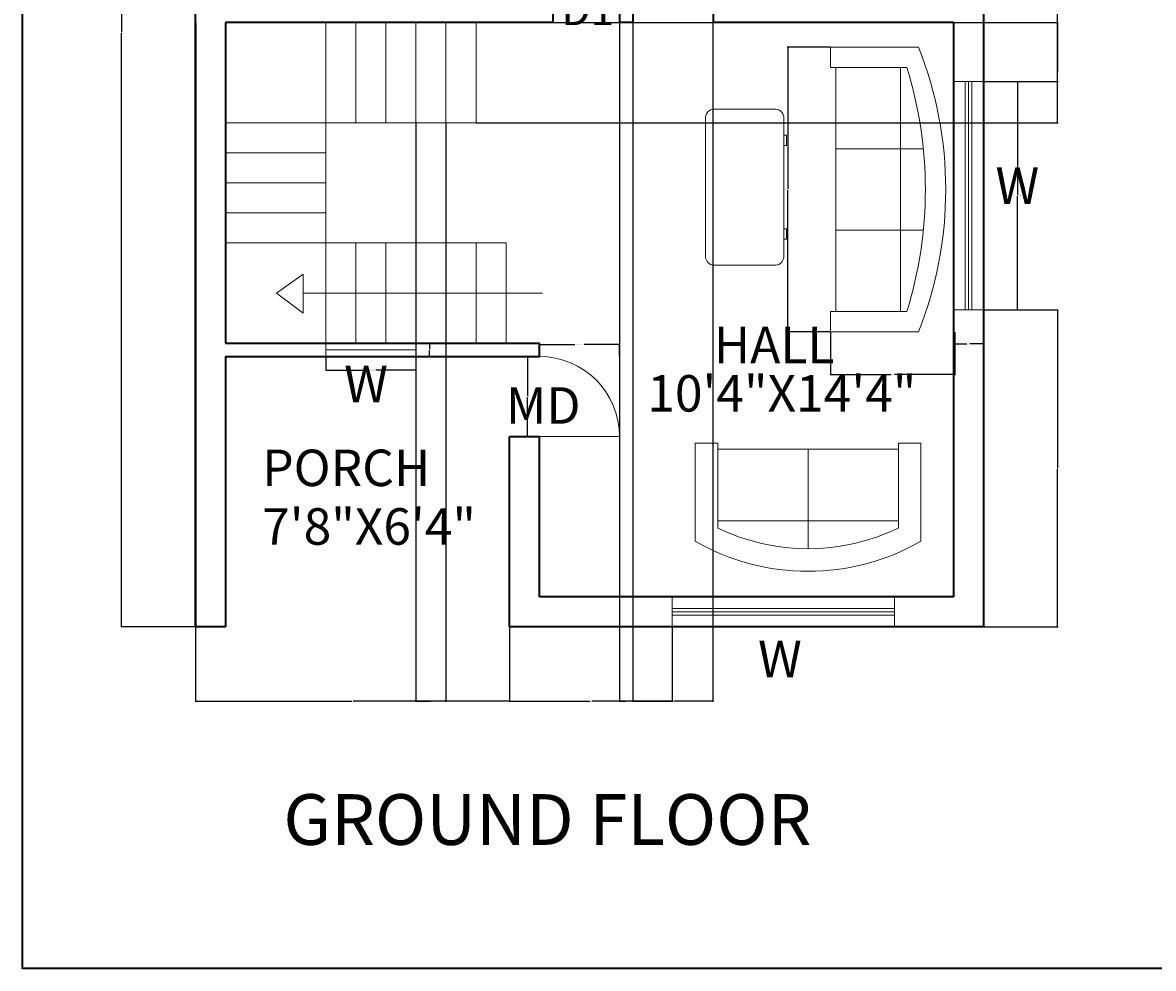
# Model space of a CAD drawing. Units: feet. Extents: x 38163 to 38841, y 65807 to 66292.
# Tile 1 of 3: x 38163 to 38502, y 65807 to 66090. Entities that reach past the tile are written whole.
import ezdxf

# ---------------------------------------------------------------- set-up
doc = ezdxf.new("R2010")
doc.units = ezdxf.units.FT
for name, color, linetype, lineweight in [('A-ANNO-DIMS', 2, 'Continuous', 18), ('A-ANNO-SYMB', 7, 'Continuous', 13), ('A-ANNO-TEXT', 7, 'Continuous', 18), ('A-ANNO-TITL', 7, 'Continuous', 25), ('A-ANNO-TTLB', 7, 'Continuous', 35), ('A-AREA-IDEN', 7, 'Continuous', 18), ('A-DOOR', 4, 'Continuous', 18), ('A-FLOR-STRS', 7, 'Continuous', 18), ('A-FURN', 8, 'Continuous', 18), ('A-GLAZ', 4, 'Continuous', 13), ('A-WALL', 7, 'Continuous', 35)]:
    doc.layers.add(name, color=color, linetype=linetype, lineweight=lineweight)
doc.styles.get("Standard").update_dxf_attribs({"font": 'arial.ttf'})
doc.dimstyles.get("Standard").update_dxf_attribs({"dimtxt": 0.18, "dimasz": 0.18, "dimexe": 0.18, "dimexo": 0.0625, "dimgap": 0.09, "dimtad": 0, "dimtih": 1, "dimtoh": 1, "dimdec": 4, "dimzin": 0, "dimdsep": 46, "dimtxsty": 'Standard', "dimcen": 0.09, "dimadec": 0, "dimazin": 0, "dimtfac": 1, "dimtdec": 4, "dimtofl": 0, "dimtmove": 0, "dimatfit": 3, "dimfxl": 1, "dimtolj": 1, "dimtzin": 0, "dimarcsym": 0})

# ---------------------------------------------------------------- blocks, each defined once
blk = doc.blocks.new('Desk - 30 x 60 in.')
for p, q in [((-26.999995, 0), (26.999995, 0)), ((-29.999995, -27), (-29.999995, -3)), ((29.999995, -3), (29.999995, -27)), ((26.999995, -30), (-26.999995, -30)), ((-20.000005, -30), (-20.000005, -31)), ((-16.000005, -31), (-16.000005, -30)), ((15.999995, -31), (15.999995, -30)), ((19.999995, -30), (19.999995, -31)), ((-20.000005, -31), (-16.000005, -31)), ((19.999995, -31), (15.999995, -31))]:
    blk.add_line(p, q)
for centre, start, end in [((-26.499995, -3.5), 98.1301, 171.8699), ((26.499995, -3.5), 8.130102, 81.8699), ((-26.499995, -26.5), 188.1301, 261.8699), ((26.499995, -26.5), 278.1301, 351.8699)]:
    blk.add_arc(centre, 3.535534, start, end)
blk = doc.blocks.new('Sofa - Roundback 7 ft.')
for p, q in [((-12.00002, -32.4421), (-12.00003, -6.5971)), ((11.99997, -32.4421), (11.99998, -6.5971)), ((-36.000027, -34), (-36.000027, -11.4696)), ((35.99998, -34), (35.99998, -11.4696)), ((-35.999844, -13.3819), (35.9998, -13.3819)), ((-36.000027, -32.4421), (35.99998, -32.4421))]:
    blk.add_line(p, q)
for points in [[(-36.000027, -34), (-42.000027, -34), (-42.000027, -8)], [(41.99998, -8), (41.99998, -34), (35.99998, -34)]]:
    blk.add_lwpolyline(points)
for centre, radius, start, end in [((0, -114.25), 114.25, 68.43141, 111.5686), ((-0.00001, -127.1968), 121.1968, 72.72033, 107.2797)]:
    blk.add_arc(centre, radius, start, end)
blk = doc.blocks.new('Sofa - Roundback Loveseat 5 ft.')
for p, q in [((0, -32.44198), (0, -5.99998)), ((-24, -33.99998), (-24, -11.46958)), ((24.00004, -33.99998), (24.00004, -11.46958)), ((-23.9998, -13.38178), (23.99986, -13.38178)), ((-24, -32.44198), (24.00004, -32.44198))]:
    blk.add_line(p, q)
for points in [[(-24, -33.99998), (-30, -33.99998), (-30, -7.99998)], [(30.00004, -7.99998), (30.00004, -33.99998), (24.00004, -33.99998)]]:
    blk.add_lwpolyline(points)
for centre, radius, start, end in [((0, -60.24998), 60.24998, 60.13715, 119.8628), ((0, -61.38438), 55.38444, 64.32083, 115.6792)]:
    blk.add_arc(centre, radius, start, end)
blk = doc.blocks.new('DOOR-SWING-24')
blk.add_line((0, 0), (24, 0))
blk.add_arc((0, 0), 24, 0, 90)
blk = doc.blocks.new('STAIR-HALF-TURN')
for p, q in [((30, 96), (30, 0)), ((39, 96), (39, 66)), ((48, 96), (48, 66)), ((57, 96), (57, 66)), ((66, 96), (66, 66)), ((75, 96), (75, 66)), ((75, 66), (0, 66)), ((30, 57), (0, 57)), ((30, 48), (0, 48)), ((30, 39), (0, 39)), ((0, 30), (84, 30)), ((39, 30), (39, 0)), ((48, 30), (48, 0)), ((57, 30), (57, 0)), ((66, 30), (66, 0)), ((75, 30), (75, 0)), ((84, 30), (84, 0))]:
    blk.add_line(p, q)
blk = doc.blocks.new('WIN-FRONT-HALL')
for p, q in [((0, 9), (0, 0)), ((66.57, 9), (66.57, 0)), ((0, 5.5), (66.57, 5.5)), ((0, 4.5), (66.57, 4.5)), ((0, 3.5), (66.57, 3.5))]:
    blk.add_line(p, q)
blk = doc.blocks.new('WIN-SIDE-HALL')
for p, q in [((0, 68.38), (9, 68.38)), ((3.5, 68.38), (3.5, 0)), ((4.5, 68.38), (4.5, 0)), ((5.5, 68.38), (5.5, 0)), ((0, 0), (9, 0))]:
    blk.add_line(p, q)
blk = doc.blocks.new('WIN-STAIR')
for p, q in [((0, 4), (0, 0)), ((27, 4), (27, 0)), ((0, 2), (27, 2))]:
    blk.add_line(p, q)
blk = doc.blocks.new('STAIR-ARROWHEAD')
for p, q in [((0, 6), (8, 11.63)), ((8, 6), (8, 11.63)), ((0, 6), (8, 0)), ((8, 6), (8, 0)), ((8, 0), (8, 0))]:
    blk.add_line(p, q)
blk = doc.blocks.new('*D23')
at = {"layer": 'A-ANNO-DIMS', "color": 0, "lineweight": -2, "transparency": 16777216}
for p, q in [((38318.09, 65990.08), (38318.09, 65993.79)), ((38318.27, 65993.61), (38328.7, 65993.61)), ((38341.91, 65993.61), (38331.49, 65993.61)), ((38342.09, 65990.08), (38342.09, 65993.79))]:
    blk.add_line(p, q, dxfattribs=at)
at = {"layer": 'A-ANNO-DIMS', "color": 0, "transparency": 16777216}
for points in [[(38318.27, 65993.64), (38318.27, 65993.58), (38318.09, 65993.61)], [(38341.91, 65993.64), (38341.91, 65993.58), (38342.09, 65993.61)]]:
    blk.add_solid(points, dxfattribs=at)
at = {"layer": 'Defpoints', "color": 0, "transparency": 16777216}
for p in [(38342.09, 65993.61), (38318.09, 65990.01), (38342.09, 65990.01)]:
    blk.add_point(p, dxfattribs=at)
at = {"layer": 'A-ANNO-DIMS', "color": 0, "transparency": 16777216, "insert": (38330.09, 65993.61), "char_height": 0.18, "attachment_point": 5}
blk.add_mtext('\\A1;ENTRY DOOR 24 TYP.', dxfattribs=at)
blk = doc.blocks.new('*D24')
at = {"layer": 'A-ANNO-DIMS', "color": 0, "lineweight": -2, "transparency": 16777216}
for p, q in [((38318.03, 65990.01), (38314.31, 65990.01)), ((38314.49, 65989.83), (38314.49, 65978.19)), ((38314.49, 65966.19), (38314.49, 65977.83)), ((38318.03, 65966.01), (38314.31, 65966.01))]:
    blk.add_line(p, q, dxfattribs=at)
at = {"layer": 'A-ANNO-DIMS', "color": 0, "transparency": 16777216}
for points in [[(38314.46, 65989.83), (38314.52, 65989.83), (38314.49, 65990.01)], [(38314.46, 65966.19), (38314.52, 65966.19), (38314.49, 65966.01)]]:
    blk.add_solid(points, dxfattribs=at)
at = {"layer": 'Defpoints', "color": 0, "transparency": 16777216}
for p in [(38314.49, 65990.01), (38318.09, 65990.01), (38318.09, 65966.01)]:
    blk.add_point(p, dxfattribs=at)
at = {"layer": 'A-ANNO-DIMS', "color": 0, "transparency": 16777216, "insert": (38314.49, 65978.01), "char_height": 0.18, "attachment_point": 5}
blk.add_mtext('\\A1;24 TYP.', dxfattribs=at)
blk = doc.blocks.new('*D31')
at = {"layer": 'A-ANNO-DIMS', "color": 0, "lineweight": -2, "transparency": 16777216}
for p, q in [((38405.21, 66082.68), (38392.3, 66082.68)), ((38392.48, 66082.5), (38392.48, 66040.2)), ((38392.48, 65997.54), (38392.48, 66039.84)), ((38405.21, 65997.36), (38392.3, 65997.36))]:
    blk.add_line(p, q, dxfattribs=at)
at = {"layer": 'A-ANNO-DIMS', "color": 0, "transparency": 16777216}
for points in [[(38392.45, 66082.5), (38392.51, 66082.5), (38392.48, 66082.68)], [(38392.45, 65997.54), (38392.51, 65997.54), (38392.48, 65997.36)]]:
    blk.add_solid(points, dxfattribs=at)
at = {"layer": 'Defpoints', "color": 0, "transparency": 16777216}
for p in [(38405.27, 66082.68), (38392.48, 65997.36), (38405.27, 65997.36)]:
    blk.add_point(p, dxfattribs=at)
at = {"layer": 'A-ANNO-DIMS', "color": 0, "transparency": 16777216, "insert": (38392.48, 66040.02), "char_height": 0.18, "attachment_point": 5}
blk.add_mtext('\\A1;SOFA 85 TYP.', dxfattribs=at)
blk = doc.blocks.new('*D32')
at = {"layer": 'A-ANNO-DIMS', "color": 0, "lineweight": -2, "transparency": 16777216}
for p, q in [((38405.27, 65997.3), (38405.27, 65984.39)), ((38442.52, 65997.3), (38442.52, 65984.39)), ((38405.45, 65984.57), (38423.37, 65984.57)), ((38442.34, 65984.57), (38424.42, 65984.57))]:
    blk.add_line(p, q, dxfattribs=at)
at = {"layer": 'A-ANNO-DIMS', "color": 0, "transparency": 16777216}
for points in [[(38405.45, 65984.6), (38405.45, 65984.54), (38405.27, 65984.57)], [(38442.34, 65984.6), (38442.34, 65984.54), (38442.52, 65984.57)]]:
    blk.add_solid(points, dxfattribs=at)
at = {"layer": 'Defpoints', "color": 0, "transparency": 16777216}
for p in [(38405.27, 65997.36), (38442.52, 65997.36), (38442.52, 65984.57)]:
    blk.add_point(p, dxfattribs=at)
at = {"layer": 'A-ANNO-DIMS', "color": 0, "transparency": 16777216, "insert": (38423.89, 65984.57), "char_height": 0.18, "attachment_point": 5}
blk.add_mtext('\\A1;37 TYP.', dxfattribs=at)
blk = doc.blocks.new('*D43')
at = {"layer": 'A-ANNO-DIMS', "color": 0, "lineweight": -2, "transparency": 16777216}
for p, q in [((38451.15, 66072.39), (38461.53, 66072.39)), ((38461.35, 66072.21), (38461.35, 66038.39)), ((38461.35, 66004.19), (38461.35, 66038.02)), ((38451.15, 66004.01), (38461.53, 66004.01))]:
    blk.add_line(p, q, dxfattribs=at)
at = {"layer": 'A-ANNO-DIMS', "color": 0, "transparency": 16777216}
for points in [[(38461.32, 66072.21), (38461.38, 66072.21), (38461.35, 66072.39)], [(38461.32, 66004.19), (38461.38, 66004.19), (38461.35, 66004.01)]]:
    blk.add_solid(points, dxfattribs=at)
at = {"layer": 'Defpoints', "color": 0, "transparency": 16777216}
for p in [(38451.09, 66072.39), (38461.35, 66072.39), (38451.09, 66004.01)]:
    blk.add_point(p, dxfattribs=at)
at = {"layer": 'A-ANNO-DIMS', "color": 0, "transparency": 16777216, "insert": (38461.35, 66038.2), "char_height": 0.18, "attachment_point": 5}
blk.add_mtext('\\A1;HALL WINDOW 68 TYP.', dxfattribs=at)
blk = doc.blocks.new('*D44')
at = {"layer": 'A-ANNO-DIMS', "color": 0, "lineweight": -2, "transparency": 16777216}
for p, q in [((38442.09, 66003.95), (38442.09, 65993.58)), ((38451.09, 66003.95), (38451.09, 65993.58)), ((38442.27, 65993.76), (38446.13, 65993.76)), ((38450.91, 65993.76), (38447.05, 65993.76))]:
    blk.add_line(p, q, dxfattribs=at)
at = {"layer": 'A-ANNO-DIMS', "color": 0, "transparency": 16777216}
for points in [[(38442.27, 65993.79), (38442.27, 65993.73), (38442.09, 65993.76)], [(38450.91, 65993.79), (38450.91, 65993.73), (38451.09, 65993.76)]]:
    blk.add_solid(points, dxfattribs=at)
at = {"layer": 'Defpoints', "color": 0, "transparency": 16777216}
for p in [(38442.09, 66004.01), (38451.09, 66004.01), (38451.09, 65993.76)]:
    blk.add_point(p, dxfattribs=at)
at = {"layer": 'A-ANNO-DIMS', "color": 0, "transparency": 16777216, "insert": (38446.59, 65993.76), "char_height": 0.18, "attachment_point": 5}
blk.add_mtext('\\A1;9 TYP.', dxfattribs=at)
blk = doc.blocks.new('*D47')
at = {"layer": 'A-ANNO-DIMS', "color": 0, "lineweight": -2, "transparency": 16777216}
for p, q in [((38254.09, 65989.95), (38254.09, 65985.78)), ((38281.09, 65989.95), (38281.09, 65985.78)), ((38254.27, 65985.96), (38266.07, 65985.96)), ((38280.91, 65985.96), (38269.11, 65985.96))]:
    blk.add_line(p, q, dxfattribs=at)
at = {"layer": 'A-ANNO-DIMS', "color": 0, "transparency": 16777216}
for points in [[(38254.27, 65985.99), (38254.27, 65985.93), (38254.09, 65985.96)], [(38280.91, 65985.99), (38280.91, 65985.93), (38281.09, 65985.96)]]:
    blk.add_solid(points, dxfattribs=at)
at = {"layer": 'Defpoints', "color": 0, "transparency": 16777216}
for p in [(38254.09, 65990.01), (38281.09, 65990.01), (38281.09, 65985.96)]:
    blk.add_point(p, dxfattribs=at)
at = {"layer": 'A-ANNO-DIMS', "color": 0, "transparency": 16777216, "insert": (38267.59, 65985.96), "char_height": 0.18, "attachment_point": 5}
blk.add_mtext('\\A1;STAIR WINDOW 27 TYP.', dxfattribs=at)
blk = doc.blocks.new('*D48')
at = {"layer": 'A-ANNO-DIMS', "color": 0, "lineweight": -2, "transparency": 16777216}
for p, q in [((38281.15, 65994.01), (38285.32, 65994.01)), ((38285.14, 65993.83), (38285.14, 65992.19)), ((38285.14, 65990.19), (38285.14, 65991.83)), ((38281.15, 65990.01), (38285.32, 65990.01))]:
    blk.add_line(p, q, dxfattribs=at)
at = {"layer": 'A-ANNO-DIMS', "color": 0, "transparency": 16777216}
for points in [[(38285.11, 65993.83), (38285.17, 65993.83), (38285.14, 65994.01)], [(38285.11, 65990.19), (38285.17, 65990.19), (38285.14, 65990.01)]]:
    blk.add_solid(points, dxfattribs=at)
at = {"layer": 'Defpoints', "color": 0, "transparency": 16777216}
for p in [(38281.09, 65994.01), (38285.14, 65994.01), (38281.09, 65990.01)]:
    blk.add_point(p, dxfattribs=at)
at = {"layer": 'A-ANNO-DIMS', "color": 0, "transparency": 16777216, "insert": (38285.14, 65992.01), "char_height": 0.18, "attachment_point": 5}
blk.add_mtext('\\A1;4 TYP.', dxfattribs=at)
blk = doc.blocks.new('*D58')
at = {"layer": 'A-ANNO-DIMS', "color": 0, "lineweight": -2, "transparency": 16777216}
for p, q in [((38215.03, 66265.01), (38192.66, 66265.01)), ((38192.84, 66264.83), (38192.84, 66087.19)), ((38192.84, 65909.19), (38192.84, 66086.83)), ((38215.03, 65909.01), (38192.66, 65909.01))]:
    blk.add_line(p, q, dxfattribs=at)
at = {"layer": 'A-ANNO-DIMS', "color": 0, "transparency": 16777216}
for points in [[(38192.81, 66264.83), (38192.87, 66264.83), (38192.84, 66265.01)], [(38192.81, 65909.19), (38192.87, 65909.19), (38192.84, 65909.01)]]:
    blk.add_solid(points, dxfattribs=at)
at = {"layer": 'Defpoints', "color": 0, "transparency": 16777216}
for p in [(38192.84, 66265.01), (38215.09, 66265.01), (38215.09, 65909.01)]:
    blk.add_point(p, dxfattribs=at)
at = {"layer": 'A-ANNO-DIMS', "color": 0, "transparency": 16777216, "insert": (38192.84, 66087.01), "char_height": 0.18, "attachment_point": 5}
blk.add_mtext('\\A1;356', dxfattribs=at)
blk = doc.blocks.new('*D61')
at = {"layer": 'A-ANNO-DIMS', "color": 0, "lineweight": -2, "transparency": 16777216}
for p, q in [((38215.09, 65908.95), (38215.09, 65886.58)), ((38309.09, 65908.95), (38309.09, 65886.58)), ((38215.27, 65886.76), (38261.87, 65886.76)), ((38308.91, 65886.76), (38262.31, 65886.76))]:
    blk.add_line(p, q, dxfattribs=at)
at = {"layer": 'A-ANNO-DIMS', "color": 0, "transparency": 16777216}
for points in [[(38215.27, 65886.79), (38215.27, 65886.73), (38215.09, 65886.76)], [(38308.91, 65886.79), (38308.91, 65886.73), (38309.09, 65886.76)]]:
    blk.add_solid(points, dxfattribs=at)
at = {"layer": 'Defpoints', "color": 0, "transparency": 16777216}
for p in [(38215.09, 65909.01), (38309.09, 65909.01), (38309.09, 65886.76)]:
    blk.add_point(p, dxfattribs=at)
at = {"layer": 'A-ANNO-DIMS', "color": 0, "transparency": 16777216, "insert": (38262.09, 65886.76), "char_height": 0.18, "attachment_point": 5}
blk.add_mtext('\\A1;94', dxfattribs=at)
blk = doc.blocks.new('*D62')
at = {"layer": 'A-ANNO-DIMS', "color": 0, "lineweight": -2, "transparency": 16777216}
for p, q in [((38309.09, 65908.95), (38309.09, 65886.58)), ((38357.89, 65908.95), (38357.89, 65886.58)), ((38309.27, 65886.76), (38333.16, 65886.76)), ((38357.71, 65886.76), (38333.82, 65886.76))]:
    blk.add_line(p, q, dxfattribs=at)
at = {"layer": 'A-ANNO-DIMS', "color": 0, "transparency": 16777216}
for points in [[(38309.27, 65886.79), (38309.27, 65886.73), (38309.09, 65886.76)], [(38357.71, 65886.79), (38357.71, 65886.73), (38357.89, 65886.76)]]:
    blk.add_solid(points, dxfattribs=at)
at = {"layer": 'Defpoints', "color": 0, "transparency": 16777216}
for p in [(38309.09, 65909.01), (38357.89, 65909.01), (38357.89, 65886.76)]:
    blk.add_point(p, dxfattribs=at)
at = {"layer": 'A-ANNO-DIMS', "color": 0, "transparency": 16777216, "insert": (38333.49, 65886.76), "char_height": 0.18, "attachment_point": 5}
blk.add_mtext('\\A1;48.8', dxfattribs=at)
blk = doc.blocks.new('*D63')
at = {"layer": 'A-ANNO-DIMS', "color": 0, "lineweight": -2, "transparency": 16777216}
for p, q in [((38451.15, 66004.01), (38473.52, 66004.01)), ((38473.34, 66003.83), (38473.34, 65956.69)), ((38473.34, 65909.19), (38473.34, 65956.33)), ((38451.15, 65909.01), (38473.52, 65909.01))]:
    blk.add_line(p, q, dxfattribs=at)
at = {"layer": 'A-ANNO-DIMS', "color": 0, "transparency": 16777216}
for points in [[(38473.31, 66003.83), (38473.37, 66003.83), (38473.34, 66004.01)], [(38473.31, 65909.19), (38473.37, 65909.19), (38473.34, 65909.01)]]:
    blk.add_solid(points, dxfattribs=at)
at = {"layer": 'Defpoints', "color": 0, "transparency": 16777216}
for p in [(38451.09, 66004.01), (38473.34, 66004.01), (38451.09, 65909.01)]:
    blk.add_point(p, dxfattribs=at)
at = {"layer": 'A-ANNO-DIMS', "color": 0, "transparency": 16777216, "insert": (38473.34, 65956.51), "char_height": 0.18, "attachment_point": 5}
blk.add_mtext('\\A1;95', dxfattribs=at)
blk = doc.blocks.new('*D64')
at = {"layer": 'A-ANNO-DIMS', "color": 0, "lineweight": -2, "transparency": 16777216}
for p, q in [((38451.15, 66132.54), (38473.52, 66132.54)), ((38473.34, 66132.36), (38473.34, 66102.65)), ((38473.34, 66072.57), (38473.34, 66102.29)), ((38451.15, 66072.39), (38473.52, 66072.39))]:
    blk.add_line(p, q, dxfattribs=at)
at = {"layer": 'A-ANNO-DIMS', "color": 0, "transparency": 16777216}
for points in [[(38473.31, 66132.36), (38473.37, 66132.36), (38473.34, 66132.54)], [(38473.31, 66072.57), (38473.37, 66072.57), (38473.34, 66072.39)]]:
    blk.add_solid(points, dxfattribs=at)
at = {"layer": 'Defpoints', "color": 0, "transparency": 16777216}
for p in [(38451.09, 66132.54), (38473.34, 66132.54), (38451.09, 66072.39)]:
    blk.add_point(p, dxfattribs=at)
at = {"layer": 'A-ANNO-DIMS', "color": 0, "transparency": 16777216, "insert": (38473.34, 66102.47), "char_height": 0.18, "attachment_point": 5}
blk.add_mtext('\\A1;60.15', dxfattribs=at)
blk = doc.blocks.new('*D68')
at = {"layer": 'A-ANNO-DIMS', "color": 0, "lineweight": -2, "transparency": 16777216}
for p, q in [((38346.09, 66089.95), (38346.09, 65886.58)), ((38370.09, 66089.95), (38370.09, 65886.58)), ((38346.27, 65886.76), (38357.87, 65886.76)), ((38369.91, 65886.76), (38358.31, 65886.76))]:
    blk.add_line(p, q, dxfattribs=at)
at = {"layer": 'A-ANNO-DIMS', "color": 0, "transparency": 16777216}
for points in [[(38346.27, 65886.79), (38346.27, 65886.73), (38346.09, 65886.76)], [(38369.91, 65886.79), (38369.91, 65886.73), (38370.09, 65886.76)]]:
    blk.add_solid(points, dxfattribs=at)
at = {"layer": 'Defpoints', "color": 0, "transparency": 16777216}
for p in [(38346.09, 66090.01), (38370.09, 66090.01), (38370.09, 65886.76)]:
    blk.add_point(p, dxfattribs=at)
at = {"layer": 'A-ANNO-DIMS', "color": 0, "transparency": 16777216, "insert": (38358.09, 65886.76), "char_height": 0.18, "attachment_point": 5}
blk.add_mtext('\\A1;24', dxfattribs=at)
blk = doc.blocks.new('*D73')
at = {"layer": 'A-ANNO-DIMS', "color": 0, "lineweight": -2, "transparency": 16777216}
for p, q in [((38299.15, 66090.01), (38473.52, 66090.01)), ((38473.34, 66089.83), (38473.34, 66075.19)), ((38473.34, 66060.19), (38473.34, 66074.83)), ((38299.15, 66060.01), (38473.52, 66060.01))]:
    blk.add_line(p, q, dxfattribs=at)
at = {"layer": 'A-ANNO-DIMS', "color": 0, "transparency": 16777216}
for points in [[(38473.31, 66089.83), (38473.37, 66089.83), (38473.34, 66090.01)], [(38473.31, 66060.19), (38473.37, 66060.19), (38473.34, 66060.01)]]:
    blk.add_solid(points, dxfattribs=at)
at = {"layer": 'Defpoints', "color": 0, "transparency": 16777216}
for p in [(38299.09, 66090.01), (38473.34, 66090.01), (38299.09, 66060.01)]:
    blk.add_point(p, dxfattribs=at)
at = {"layer": 'A-ANNO-DIMS', "color": 0, "transparency": 16777216, "insert": (38473.34, 66075.01), "char_height": 0.18, "attachment_point": 5}
blk.add_mtext('\\A1;30', dxfattribs=at)
blk = doc.blocks.new('*D74')
at = {"layer": 'A-ANNO-DIMS', "color": 0, "lineweight": -2, "transparency": 16777216}
for p, q in [((38281.09, 66059.95), (38281.09, 65886.58)), ((38290.09, 66059.95), (38290.09, 65886.58)), ((38281.27, 65886.76), (38285.44, 65886.76)), ((38289.91, 65886.76), (38285.74, 65886.76))]:
    blk.add_line(p, q, dxfattribs=at)
at = {"layer": 'A-ANNO-DIMS', "color": 0, "transparency": 16777216}
for points in [[(38281.27, 65886.79), (38281.27, 65886.73), (38281.09, 65886.76)], [(38289.91, 65886.79), (38289.91, 65886.73), (38290.09, 65886.76)]]:
    blk.add_solid(points, dxfattribs=at)
at = {"layer": 'Defpoints', "color": 0, "transparency": 16777216}
for p in [(38281.09, 66060.01), (38290.09, 66060.01), (38290.09, 65886.76)]:
    blk.add_point(p, dxfattribs=at)
at = {"layer": 'A-ANNO-DIMS', "color": 0, "transparency": 16777216, "insert": (38285.59, 65886.76), "char_height": 0.18, "attachment_point": 5}
blk.add_mtext('\\A1;9', dxfattribs=at)
blk = doc.blocks.new('*D80')
at = {"layer": 'A-ANNO-DIMS', "color": 0, "lineweight": -2, "transparency": 16777216}
for p, q in [((38342.09, 66255.95), (38342.09, 65886.58)), ((38346.09, 66255.95), (38346.09, 65886.58)), ((38342.27, 65886.76), (38343.94, 65886.76)), ((38345.91, 65886.76), (38344.24, 65886.76))]:
    blk.add_line(p, q, dxfattribs=at)
at = {"layer": 'A-ANNO-DIMS', "color": 0, "transparency": 16777216}
for points in [[(38342.27, 65886.79), (38342.27, 65886.73), (38342.09, 65886.76)], [(38345.91, 65886.79), (38345.91, 65886.73), (38346.09, 65886.76)]]:
    blk.add_solid(points, dxfattribs=at)
at = {"layer": 'Defpoints', "color": 0, "transparency": 16777216}
for p in [(38342.09, 66256.01), (38346.09, 66256.01), (38346.09, 65886.76)]:
    blk.add_point(p, dxfattribs=at)
at = {"layer": 'A-ANNO-DIMS', "color": 0, "transparency": 16777216, "insert": (38344.09, 65886.76), "char_height": 0.18, "attachment_point": 5}
blk.add_mtext('\\A1;4', dxfattribs=at)

msp = doc.modelspace()

# ---------------------------------------------------------------- linework, layer by layer
at = {"layer": 'A-ANNO-SYMB'}
msp.add_line((38247.284, 66009.006), (38319.045, 66009.006), dxfattribs=at)
at = {"layer": 'A-ANNO-TTLB'}
msp.add_lwpolyline([(38163.261, 66292.238), (38840.784, 66292.238), (38840.784, 65806.731), (38163.261, 65806.731)], close=True, dxfattribs=at)
at = {"layer": 'A-WALL'}
for p, q in [((38215.092, 65909.013), (38215.092, 66265.013)), ((38451.092, 66265.013), (38451.092, 65909.013)), ((38342.092, 66256.013), (38342.092, 66090.013)), ((38346.092, 66256.013), (38346.092, 66090.013)), ((38322.092, 66094.013), (38322.092, 66090.013)), ((38370.092, 66094.013), (38370.092, 66090.013)), ((38215.092, 66090.013), (38215.092, 65909.013)), ((38322.092, 66090.013), (38224.092, 66090.013)), ((38224.092, 66090.013), (38224.092, 65994.013)), ((38322.092, 66090.013), (38224.092, 66090.013)), ((38346.092, 66090.013), (38342.092, 66090.013)), ((38442.092, 66090.013), (38370.092, 66090.013)), ((38442.092, 66090.013), (38442.092, 65918.013)), ((38442.092, 66090.013), (38442.092, 66071.969)), ((38451.092, 66090.013), (38451.092, 65909.013)), ((38224.092, 65994.013), (38318.092, 65994.013)), ((38318.092, 65990.013), (38318.092, 65994.013)), ((38224.092, 65990.013), (38318.092, 65990.013)), ((38224.092, 65990.013), (38224.092, 65909.013)), ((38309.092, 65909.013), (38309.092, 65966.013)), ((38309.092, 65966.013), (38318.092, 65966.013)), ((38318.092, 65918.013), (38318.092, 65966.013)), ((38442.092, 65918.013), (38318.092, 65918.013)), ((38224.092, 65909.013), (38215.092, 65909.013)), ((38451.092, 65909.013), (38309.092, 65909.013))]:
    msp.add_line(p, q, dxfattribs=at)

# ---------------------------------------------------------------- block references
at = {"layer": 'A-ANNO-SYMB'}
msp.add_blockref('STAIR-ARROWHEAD', (38239.284, 66003.006), dxfattribs=at)
at = {"layer": 'A-DOOR'}
msp.add_blockref('DOOR-SWING-24', (38318.092, 65966.013), dxfattribs=at)
at = {"layer": 'A-FLOR-STRS'}
msp.add_blockref('STAIR-HALF-TURN', (38224.092, 65994.013), dxfattribs=at)
at = {"layer": 'A-FURN'}
for name, p, xscale, yscale, zscale, rotation in [('Sofa - Roundback 7 ft.', (38439.807, 66040.021), 1.015660350660268, 1.015660350660268, 1.015660350660268, 270), ('Desk - 30 x 60 in.', (38367.876, 66040.731), 0.7801287338679669, 0.7801287338679669, 0.7801287338679669, 90), ('Sofa - Roundback Loveseat 5 ft.', (38398.558, 65925.671), 1.127499616246774, 1.127499616246774, 1.127499616246774, 180)]:
    msp.add_blockref(name, p, dxfattribs=dict(at, xscale=xscale, yscale=yscale, zscale=zscale, rotation=rotation))
at = {"layer": 'A-GLAZ'}
for name, p in [('WIN-SIDE-HALL', (38442.092, 66004.013)), ('WIN-STAIR', (38254.092, 65990.013)), ('WIN-FRONT-HALL', (38357.893, 65909.013))]:
    msp.add_blockref(name, p, dxfattribs=at)

# ---------------------------------------------------------------- texts
at = {"layer": 'A-ANNO-TEXT'}
for s, height, p in [('D1', 9.3586, (38324.641, 66089.25)), ('W', 10.93, (38454.715, 66035.707)), ('W', 10.93, (38259.609, 65976.282)), ('MD', 10.9298, (38308.049, 65969.866)), ('W', 10.93, (38383.595, 65893.929))]:
    msp.add_text(s, height=height, dxfattribs=at).set_placement(p)
at = {"layer": 'A-ANNO-TITL'}
msp.add_text('GROUND FLOOR', height=15.18709, dxfattribs=at).set_placement((38241.383, 65843.726))
at = {"layer": 'A-AREA-IDEN'}
for s, p in [('HALL', (38370.355, 65987.969)), ('10\'4"X14\'4"', (38350.4, 65973.503)), ('PORCH', (38235.024, 65951.194)), ('7\'8"X6\'4"', (38235.024, 65933.636))]:
    msp.add_text(s, height=10.9298, dxfattribs=at).set_placement(p)

# ---------------------------------------------------------------- dimensions: what is measured, and where the dimension line sits
at = {"layer": 'A-ANNO-DIMS'}
for base, p1, p2, override, picture, middle in [((38192.842, 66265.013), (38215.092, 65909.013), (38215.092, 66265.013), {"dimdec": 0, "dimlfac": 1, "dimrnd": 0, "dimzin": 0, "dimdsep": 46, "dimlunit": 2}, '*D58', (38192.842, 66087.013)), ((38473.342, 66132.544), (38451.092, 66072.393), (38451.092, 66132.544), {"dimdec": 2, "dimlfac": 1, "dimrnd": 0, "dimzin": 0, "dimdsep": 46, "dimlunit": 2}, '*D64', (38473.342, 66102.469)), ((38473.342, 66090.013), (38299.092, 66060.013), (38299.092, 66090.013), {"dimdec": 0, "dimlfac": 1, "dimrnd": 0, "dimzin": 0, "dimdsep": 46, "dimlunit": 2}, '*D73', (38473.342, 66075.013)), ((38473.342, 66004.013), (38451.092, 65909.013), (38451.092, 66004.013), {"dimdec": 0, "dimlfac": 1, "dimrnd": 0, "dimzin": 0, "dimdsep": 46, "dimlunit": 2}, '*D63', (38473.342, 65956.513))]:
    dim = msp.add_linear_dim(base=base, p1=p1, p2=p2, angle=90, dimstyle='Standard', override=override, dxfattribs=at)
    dim.commit()
    dim.dimension.update_dxf_attribs({"geometry": picture, "text_midpoint": middle})
for base, p1, p2, override, picture, middle in [((38346.092, 65886.763), (38342.092, 66256.013), (38346.092, 66256.013), {"dimdec": 0, "dimlfac": 1, "dimrnd": 0, "dimzin": 0, "dimdsep": 46, "dimlunit": 2}, '*D80', (38344.092, 65886.763)), ((38370.092, 65886.763), (38346.092, 66090.013), (38370.092, 66090.013), {"dimdec": 0, "dimlfac": 1, "dimrnd": 0, "dimzin": 0, "dimdsep": 46, "dimlunit": 2}, '*D68', (38358.092, 65886.763)), ((38290.092, 65886.763), (38281.092, 66060.013), (38290.092, 66060.013), {"dimdec": 0, "dimlfac": 1, "dimrnd": 0, "dimzin": 0, "dimdsep": 46, "dimlunit": 2}, '*D74', (38285.592, 65886.763)), ((38309.092, 65886.763), (38215.092, 65909.013), (38309.092, 65909.013), {"dimdec": 0, "dimlfac": 1, "dimrnd": 0, "dimzin": 0, "dimdsep": 46, "dimlunit": 2}, '*D61', (38262.092, 65886.763)), ((38357.893, 65886.763), (38309.092, 65909.013), (38357.893, 65909.013), {"dimdec": 1, "dimlfac": 1, "dimrnd": 0, "dimzin": 0, "dimdsep": 46, "dimlunit": 2}, '*D62', (38333.492, 65886.763))]:
    dim = msp.add_linear_dim(base=base, p1=p1, p2=p2, dimstyle='Standard', override=override, dxfattribs=at)
    dim.commit()
    dim.dimension.update_dxf_attribs({"geometry": picture, "text_midpoint": middle})
for base, p1, p2, angle, text, picture, middle in [((38392.477, 65997.363), (38405.274, 66082.678), (38405.274, 65997.363), 270, 'SOFA <> TYP.', '*D31', (38392.477, 66040.021)), ((38461.349, 66072.393), (38451.092, 66004.013), (38451.092, 66072.393), 90, 'HALL WINDOW <> TYP.', '*D43', (38461.349, 66038.203)), ((38285.142, 65994.013), (38281.092, 65990.013), (38281.092, 65994.013), 90, '<> TYP.', '*D48', (38285.142, 65992.013)), ((38314.492, 65990.013), (38318.092, 65966.013), (38318.092, 65990.013), 90, '<> TYP.', '*D24', (38314.492, 65978.013))]:
    dim = msp.add_linear_dim(base=base, p1=p1, p2=p2, angle=angle, text=text, dimstyle='Standard', override={"dimdec": 0, "dimlfac": 1, "dimrnd": 0, "dimzin": 0, "dimdsep": 46, "dimlunit": 2}, dxfattribs=at)
    dim.commit()
    dim.dimension.update_dxf_attribs({"geometry": picture, "text_midpoint": middle})
for base, p1, p2, text, picture, middle in [((38451.092, 65993.756), (38442.092, 66004.013), (38451.092, 66004.013), '<> TYP.', '*D44', (38446.592, 65993.756)), ((38342.092, 65993.613), (38318.092, 65990.013), (38342.092, 65990.013), 'ENTRY DOOR <> TYP.', '*D23', (38330.092, 65993.613)), ((38442.515, 65984.566), (38405.274, 65997.363), (38442.515, 65997.363), '<> TYP.', '*D32', (38423.895, 65984.566)), ((38281.092, 65985.963), (38254.092, 65990.013), (38281.092, 65990.013), 'STAIR WINDOW <> TYP.', '*D47', (38267.592, 65985.963))]:
    dim = msp.add_linear_dim(base=base, p1=p1, p2=p2, text=text, dimstyle='Standard', override={"dimdec": 0, "dimlfac": 1, "dimrnd": 0, "dimzin": 0, "dimdsep": 46, "dimlunit": 2}, dxfattribs=at)
    dim.commit()
    dim.dimension.update_dxf_attribs({"geometry": picture, "text_midpoint": middle})

doc.saveas('drawing.dxf')
